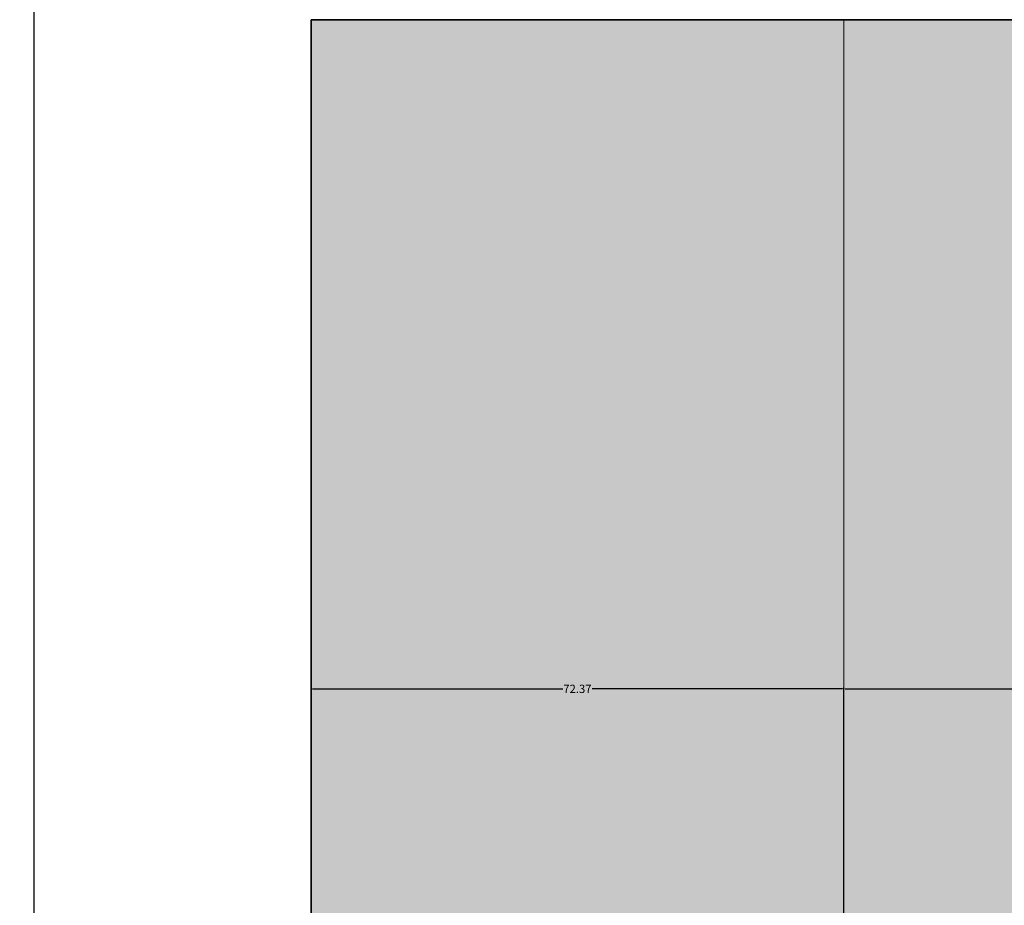
# Model space of a CAD drawing. Units: inches. Extents: x 8 to 634, y 41 to 867.
# Tile 14 of 21: x 8 to 141, y 577 to 698. Entities that reach past the tile are written whole.
import ezdxf

# ---------------------------------------------------------------- set-up
doc = ezdxf.new("R2010")
doc.units = ezdxf.units.IN
doc.header["$MEASUREMENT"] = 0
for name, color, linetype, lineweight in [('A-ANNO-DIMS', 2, 'Continuous', 18), ('A-WALL', 7, 'Continuous', 35), ('A-WALL-PANL', 7, 'Continuous', 18), ('A-WALL-PATT', 8, 'Continuous', 9)]:
    doc.layers.add(name, color=color, linetype=linetype, lineweight=lineweight)
doc.styles.get("Standard").update_dxf_attribs({"font": 'arial.ttf'})
doc.dimstyles.get("Standard").update_dxf_attribs({"dimtxt": 1.125, "dimasz": 0.18, "dimexe": 0.18, "dimexo": 0.0625, "dimgap": 0.09, "dimtad": 0, "dimtih": 1, "dimtoh": 1, "dimdec": 4, "dimzin": 0, "dimdsep": 46, "dimlunit": 4, "dimtxsty": 'Standard', "dimcen": 0.09, "dimadec": 0, "dimazin": 0, "dimtfac": 1, "dimtdec": 4, "dimtofl": 0, "dimtmove": 0, "dimatfit": 3, "dimfxl": 1, "dimtolj": 1, "dimtzin": 0, "dimarcsym": 0})

# ---------------------------------------------------------------- blocks, each defined once
blk = doc.blocks.new('*D20')
at = {"layer": 'A-ANNO-DIMS', "color": 0, "lineweight": -2, "transparency": 16777216}
for p, q in [((144.29, 828.98), (9.51, 828.98)), ((9.69, 828.8), (9.69, 454.93)), ((9.69, 79.74), (9.69, 453.6)), ((47.28, 79.56), (9.51, 79.56))]:
    blk.add_line(p, q, dxfattribs=at)
at = {"layer": 'A-ANNO-DIMS', "color": 0, "transparency": 16777216}
for points in [[(9.66, 828.8), (9.72, 828.8), (9.69, 828.98)], [(9.66, 79.74), (9.72, 79.74), (9.69, 79.56)]]:
    blk.add_solid(points, dxfattribs=at)
at = {"layer": 'Defpoints', "color": 0, "transparency": 16777216}
for p in [(9.69, 828.98), (144.36, 828.98), (47.34, 79.56)]:
    blk.add_point(p, dxfattribs=at)
at = {"layer": 'A-ANNO-DIMS', "color": 0, "transparency": 16777216, "insert": (9.69, 454.27), "char_height": 1.125, "attachment_point": 5}
blk.add_mtext('\\A1;749.4', dxfattribs=at)
blk = doc.blocks.new('*D57')
at = {"layer": 'A-ANNO-DIMS', "color": 0, "lineweight": -2, "transparency": 16777216}
for p, q in [((119.71, 569.23), (119.71, 607)), ((119.89, 606.82), (200.22, 606.82)), ((284.43, 606.82), (204.09, 606.82)), ((284.61, 569.23), (284.61, 607))]:
    blk.add_line(p, q, dxfattribs=at)
at = {"layer": 'A-ANNO-DIMS', "color": 0, "transparency": 16777216}
for points in [[(119.89, 606.85), (119.89, 606.79), (119.71, 606.82)], [(284.43, 606.85), (284.43, 606.79), (284.61, 606.82)]]:
    blk.add_solid(points, dxfattribs=at)
at = {"layer": 'Defpoints', "color": 0, "transparency": 16777216}
for p in [(284.61, 606.82), (119.71, 569.17), (284.61, 569.17)]:
    blk.add_point(p, dxfattribs=at)
at = {"layer": 'A-ANNO-DIMS', "color": 0, "transparency": 16777216, "insert": (202.16, 606.82), "char_height": 1.125, "attachment_point": 5}
blk.add_mtext('\\A1;164.9', dxfattribs=at)
blk = doc.blocks.new('*D58')
at = {"layer": 'A-ANNO-DIMS', "color": 0, "lineweight": -2, "transparency": 16777216}
for p, q in [((47.34, 569.23), (47.34, 607)), ((47.52, 606.82), (81.54, 606.82)), ((119.53, 606.82), (85.51, 606.82)), ((119.71, 569.23), (119.71, 607))]:
    blk.add_line(p, q, dxfattribs=at)
at = {"layer": 'A-ANNO-DIMS', "color": 0, "transparency": 16777216}
for points in [[(47.52, 606.85), (47.52, 606.79), (47.34, 606.82)], [(119.53, 606.85), (119.53, 606.79), (119.71, 606.82)]]:
    blk.add_solid(points, dxfattribs=at)
at = {"layer": 'Defpoints', "color": 0, "transparency": 16777216}
for p in [(119.71, 606.82), (47.34, 569.17), (119.71, 569.17)]:
    blk.add_point(p, dxfattribs=at)
at = {"layer": 'A-ANNO-DIMS', "color": 0, "transparency": 16777216, "insert": (83.52, 606.82), "char_height": 1.125, "attachment_point": 5}
blk.add_mtext('\\A1;72.37', dxfattribs=at)

msp = doc.modelspace()

# ---------------------------------------------------------------- hatches: boundary and pattern name
at = {"layer": 'A-WALL-PATT', "transparency": 33554687}
h = msp.add_hatch(dxfattribs=at)
h.set_pattern_fill('AR-CONC', color=256, scale=3.2)
h.paths.add_polyline_path([(119.7065, 697.6655), (47.3401, 697.6655), (47.3401, 569.1705), (119.7065, 569.1705)])
h.paths.add_polyline_path([(202.1558, 697.6655), (119.7065, 697.6655), (119.7065, 569.1705), (202.1558, 569.1705)])
h.paths.add_polyline_path([(284.6051, 697.6655), (202.1558, 697.6655), (202.1558, 569.1705), (284.6051, 569.1705)])
h.paths.add_polyline_path([(119.7065, 569.1705), (47.3401, 569.1705), (47.3401, 523.5555), (47.3401, 449.7533), (119.7065, 449.7533)])
h.paths.add_polyline_path([(342.6544, 682.1444), (360.785, 697.6655), (284.6051, 697.6655), (284.6051, 569.1705), (342.6544, 569.1705)])
h.paths.add_polyline_path([(342.6544, 569.1705), (284.6051, 569.1705), (284.6051, 449.7533), (342.6544, 449.7533)])
h.paths.add_polyline_path([(418.2881, 691.978), (418.2881, 697.6655), (360.785, 697.6655), (360.785, 569.1705), (418.2881, 569.1705)])
h.paths.add_polyline_path([(418.2881, 569.1705), (360.785, 569.1705), (360.785, 523.5555), (360.785, 449.7533), (418.2881, 449.7533)])
h.paths.add_polyline_path([(594.3501, 697.6655), (539.0002, 697.6655), (539.0002, 691.978), (539.0002, 569.1705), (594.3501, 569.1705)])
h.paths.add_polyline_path([(594.3501, 523.5555), (594.3501, 569.1705), (539.0002, 569.1705), (539.0002, 451.6305), (594.3501, 451.6305)])
h.paths.add_polyline_path([(594.3501, 451.6305), (539.0002, 451.6305), (539.0002, 391.7598), (594.3501, 391.7598)])
h.paths.add_polyline_path([(594.3501, 391.7598), (539.0002, 391.7598), (539.0002, 276.166), (594.3501, 276.166)])
h.paths.add_polyline_path([(418.2881, 449.7533), (360.785, 449.7533), (360.785, 391.7598), (418.2881, 391.7598)])
h.paths.add_polyline_path([(342.6544, 449.7533), (284.6051, 449.7533), (284.6051, 391.7598), (342.6544, 391.7598)])
h.paths.add_polyline_path([(342.6544, 391.7598), (284.6051, 391.7598), (284.6051, 272.3426), (342.6544, 272.3426)])
h.paths.add_polyline_path([(418.2881, 391.7598), (360.785, 391.7598), (360.785, 272.3426), (418.2881, 272.3426)])
h.paths.add_polyline_path([(418.2881, 272.3426), (360.785, 272.3426), (360.785, 235.5555), (418.2881, 235.5555)])
h.paths.add_polyline_path([(342.6544, 272.3426), (284.6051, 272.3426), (284.6051, 235.5555), (295.0049, 235.5555), (342.6544, 235.5555)])
h.paths.add_polyline_path([(594.3501, 276.166), (539.0002, 276.166), (539.0002, 228.4951), (594.3501, 228.4951)])
h.paths.add_polyline_path([(594.3501, 228.4951), (539.0002, 228.4951), (539.0002, 91.5417), (594.3501, 91.5417)])
h.paths.add_polyline_path([(418.2881, 235.5555), (360.785, 235.5555), (360.785, 91.5417), (418.2881, 91.5417)])
h.paths.add_polyline_path([(284.6051, 272.3426), (119.7065, 272.3426), (119.7065, 235.5555), (284.6051, 235.5555)])
h.paths.add_polyline_path([(119.7065, 272.3426), (47.3401, 272.3426), (47.3401, 235.5555), (47.3401, 91.5555), (63.5448, 91.5555), (63.5448, 227.8036), (268.998, 227.8036), (268.998, 91.5555), (295.0049, 91.5555), (295.0049, 222.583), (271.9787, 222.583), (271.9787, 229.0481), (62.4019, 229.0481), (62.4019, 222.583), (61.1827, 222.583), (61.1827, 235.5555), (119.7065, 235.5555)])
h.paths.add_polyline_path([(119.7065, 391.7598), (47.3401, 391.7598), (47.3401, 379.5555), (47.3401, 272.3426), (119.7065, 272.3426)])
h.paths.add_polyline_path([(119.7065, 449.7533), (47.3401, 449.7533), (47.3401, 391.7598), (119.7065, 391.7598)])
h.paths.add_polyline_path([(202.1558, 449.7533), (119.7065, 449.7533), (119.7065, 391.7598), (202.1558, 391.7598)])
h.paths.add_polyline_path([(284.6051, 449.7533), (202.1558, 449.7533), (202.1558, 391.7598), (284.6051, 391.7598)])

# ---------------------------------------------------------------- linework, layer by layer
at = {"layer": 'A-WALL'}
for p, q in [((47.3401, 523.5555), (47.3401, 697.6655)), ((47.3401, 697.6655), (360.785, 697.6655))]:
    msp.add_line(p, q, dxfattribs=at)
at = {"layer": 'A-WALL-PANL'}
msp.add_line((119.7065, 569.1705), (119.7065, 697.6655), dxfattribs=at)

# ---------------------------------------------------------------- dimensions: what is measured, and where the dimension line sits
at = {"layer": 'A-ANNO-DIMS'}
dim = msp.add_linear_dim(base=(9.6901, 828.9821), p1=(47.3401, 79.5555), p2=(144.3564, 828.9821), angle=90, dimstyle='Standard', override={"dimdec": 1, "dimlfac": 1, "dimrnd": 0, "dimzin": 0, "dimdsep": 46, "dimlunit": 2}, dxfattribs=at)
dim.commit()
dim.dimension.update_dxf_attribs({"geometry": '*D20', "text_midpoint": (9.6901, 454.2688)})
for base, p1, p2, override, picture, middle in [((119.7065, 606.8205), (47.3401, 569.1705), (119.7065, 569.1705), {"dimdec": 2, "dimlfac": 1, "dimrnd": 0, "dimzin": 0, "dimdsep": 46, "dimlunit": 2}, '*D58', (83.5233, 606.8205)), ((284.6051, 606.8205), (119.7065, 569.1705), (284.6051, 569.1705), {"dimdec": 1, "dimlfac": 1, "dimrnd": 0, "dimzin": 0, "dimdsep": 46, "dimlunit": 2}, '*D57', (202.1558, 606.8205))]:
    dim = msp.add_linear_dim(base=base, p1=p1, p2=p2, dimstyle='Standard', override=override, dxfattribs=at)
    dim.commit()
    dim.dimension.update_dxf_attribs({"geometry": picture, "text_midpoint": middle})

doc.saveas('drawing.dxf')
